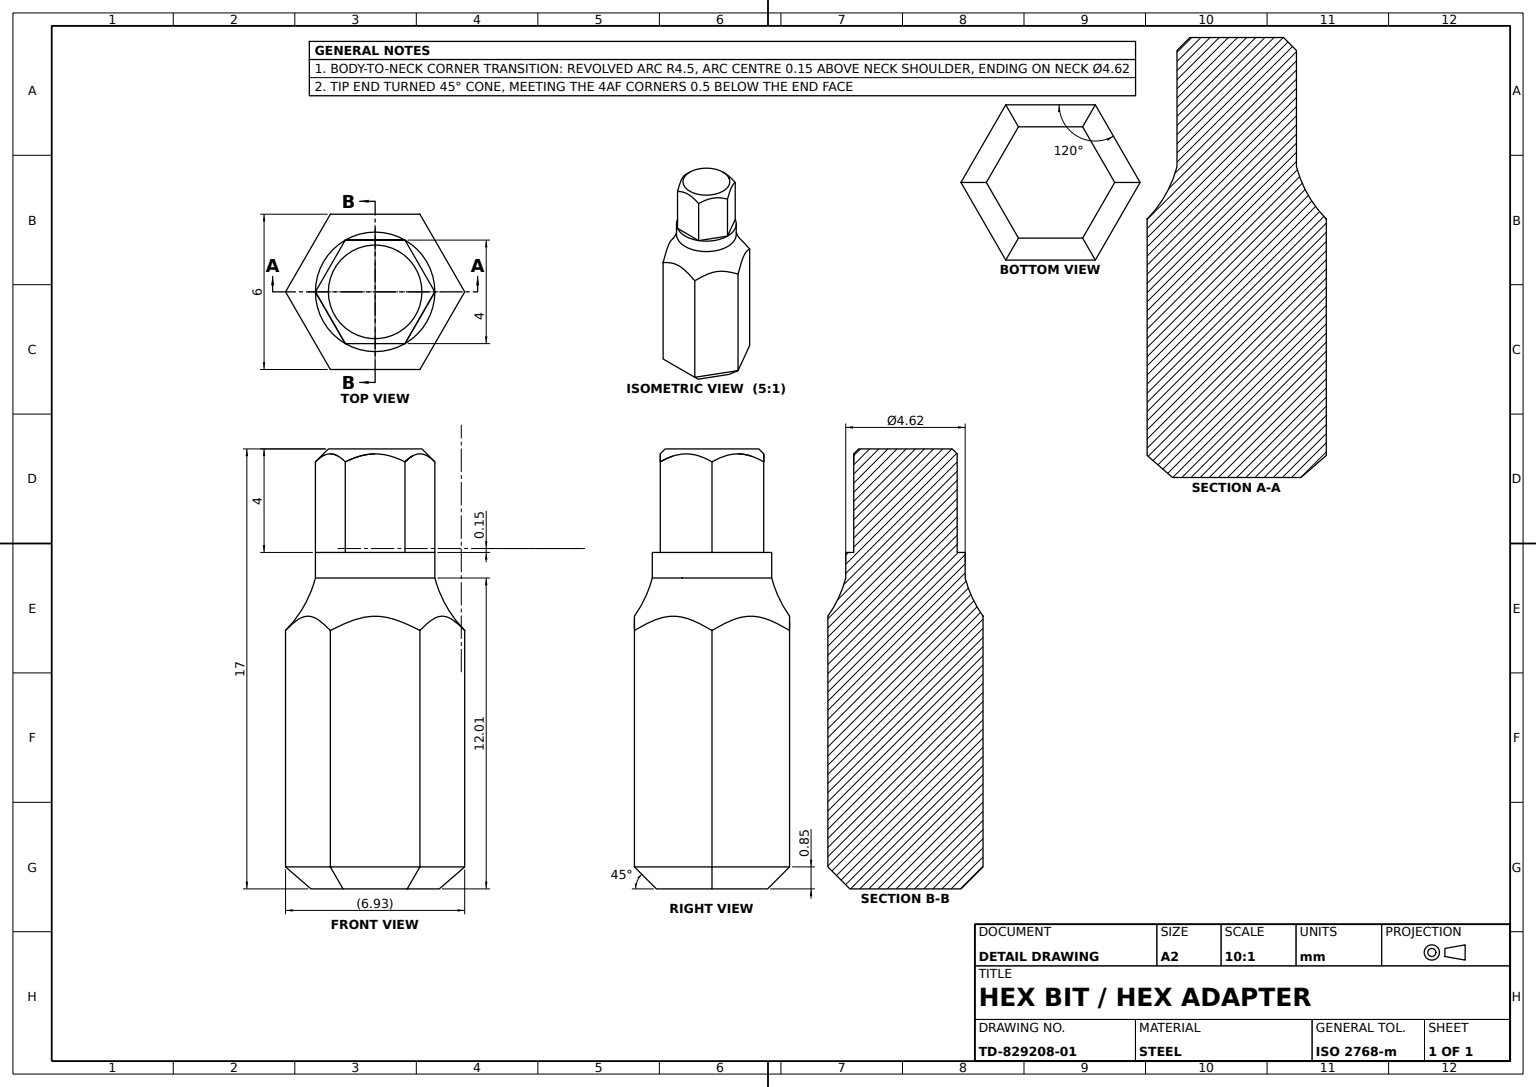
from build123d import *

# Parameters (mm, degrees)
HEX_BODY_6AF_X17_DEPTH        = 17
EDGE_CHAMFER_0_85_SIZE        = 0.85
HEX_TIP_PROFILE_4AF_OUTSIDE_W = 12.79
HEX_TIP_PROFILE_4AF_OUTSIDE_H = 11.862
HEX_TIP_4AF_X4_DEPTH          = 4


with BuildPart() as part:
    # Hex Body Profile 6AF → Hex Body 6AF x17 (new body)
    with BuildSketch(Plane(origin=(0, 0, 0), x_dir=(1, 0, 0), z_dir=(0, 1, 0))):
        Polygon((3.464101615, 0), (1.732050808, 3), (-1.732050808, 3), (-3.464101615, 0), (-1.732050808, -3), (1.732050808, -3), align=None)
    extrude(amount=HEX_BODY_6AF_X17_DEPTH)

    # Edge Chamfer 0.85
    edge_chamfer_0_85_edges = [part.edges().sort_by_distance(p)[0] for p in [
        (0, 0, 3),
        (-2.598076211, 0, 1.5),
        (-2.598076211, 0, -1.5),
        (0, 0, -3),
        (2.598076211, 0, -1.5),
        (2.598076211, 0, 1.5),
    ]]
    chamfer(edge_chamfer_0_85_edges, length=EDGE_CHAMFER_0_85_SIZE)

    # Hex Tip Profile 4AF outside → Hex Tip 4AF x4 (cut)
    with BuildSketch(Plane(origin=(0, 17, 0), x_dir=(1, 0, 0), z_dir=(0, 1, 0))):
        Rectangle(HEX_TIP_PROFILE_4AF_OUTSIDE_W, HEX_TIP_PROFILE_4AF_OUTSIDE_H)
        Polygon((2.309401077, 0), (1.154700538, 2), (-1.154700538, 2), (-2.309401077, 0), (-1.154700538, -2), (1.154700538, -2), align=None, mode=Mode.SUBTRACT)
    extrude(amount=-HEX_TIP_4AF_X4_DEPTH, mode=Mode.SUBTRACT)

    # Neck Groove Profile → Neck Groove (revolve, cut)
    with BuildSketch(Plane.XY):
        with BuildLine():
            Line((-3.464101615, 12.012038592), (-3.464101615, 13))
            Line((-3.464101615, 13), (-2.309401077, 13))
            ThreePointArc((-2.309401077, 13), (-2.659285909, 12.240164314), (-3.464101615, 12.012038592))
        make_face()
        with BuildLine():
            ThreePointArc((2.309401077, 12.012038592), (2.751182948, 10.926492222), (3.458298406, 9.991842624))
            Line((3.458298406, 9.991842624), (3.458298406, 12.012038592))
            Line((3.458298406, 12.012038592), (2.309401077, 12.012038592))
        make_face()
    revolve(axis=Axis((0, 17, 0), (0, -1, 0)), mode=Mode.SUBTRACT)

    # Hex Corner Turn Profile → Hex Corner Turn (revolve, cut)
    with BuildSketch(Plane.XY, mode=Mode.PRIVATE) as hex_corner_turn_sk:
        with BuildLine():
            Line((2.309401077, 16.837685955), (2.309401077, 13))
            Line((2.309401077, 13), (2.309401077, 12.012038592))
            ThreePointArc((2.309401077, 12.012038592), (2.751182948, 10.926492222), (3.458298406, 9.991842624))
            Line((3.458298406, 9.991842624), (11.092376237, 19.473540628))
            Line((11.092376237, 19.473540628), (2.309401077, 19.67629868))
            Line((2.309401077, 19.67629868), (2.309401077, 17))
            Line((2.309401077, 17), (2.309401077, 16.837685955))
        make_face()
    revolve(hex_corner_turn_sk.sketch.rotate(Axis((0, 0, 0), (0, 1, 0)), 179.8330498), axis=Axis((0, 0, 0), (0, 1, 0)), mode=Mode.SUBTRACT)

    # Tip Chamfer Profile → Tip Chamfer 0.5x45 (revolve, cut)
    with BuildSketch(Plane.XY, mode=Mode.PRIVATE) as tip_chamfer_0_5x45_sk:
        Polygon((-1.809401077, 17), (-2.309401077, 17), (-2.309401077, 16.5), align=None)
    revolve(tip_chamfer_0_5x45_sk.sketch.rotate(Axis((0, 17, 0), (0, -1, 0)), 90), axis=Axis((0, 17, 0), (0, -1, 0)), mode=Mode.SUBTRACT)


solid = part.part
